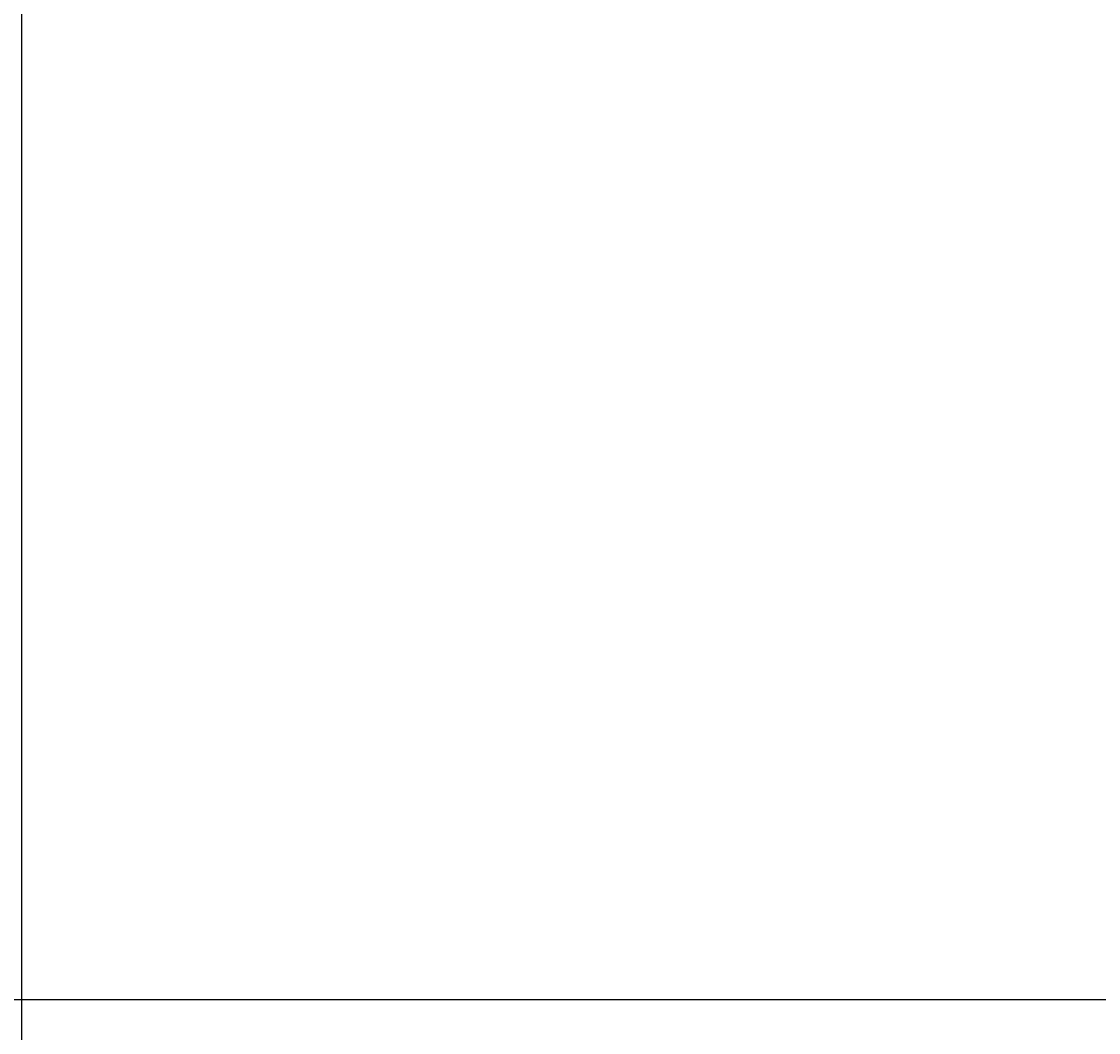
# Model space of a CAD drawing. Units: inches. Extents: x 35362 to 73946, y 43607 to 67532.
# Tile 134 of 134: x 67327 to 67834, y 59170 to 59646. Entities that reach past the tile are written whole.
import ezdxf

# ---------------------------------------------------------------- set-up
doc = ezdxf.new("R2010")
doc.units = ezdxf.units.IN
doc.header["$MEASUREMENT"] = 0
doc.layers.add('A-ANNO-DIMS', color=2, linetype='Continuous', lineweight=18)
doc.styles.get("Standard").update_dxf_attribs({"font": 'arial.ttf'})
doc.dimstyles.get("Standard").update_dxf_attribs({"dimtxt": 0.18, "dimasz": 0.18, "dimexe": 0.18, "dimexo": 0.0625, "dimgap": 0.09, "dimtad": 0, "dimtih": 1, "dimtoh": 1, "dimdec": 4, "dimzin": 0, "dimdsep": 46, "dimtxsty": 'Standard', "dimcen": 0.09, "dimadec": 0, "dimazin": 0, "dimtfac": 1, "dimtdec": 4, "dimtofl": 0, "dimtmove": 0, "dimatfit": 3, "dimfxl": 1, "dimtolj": 1, "dimtzin": 0, "dimarcsym": 0})

# ---------------------------------------------------------------- blocks, each defined once
blk = doc.blocks.new('*D8')
at = {"layer": 'A-ANNO-DIMS', "color": 0, "lineweight": -2, "transparency": 16777216}
for p, q in [((66271.28651900003, 65771.51172800003), (73945.82566600003, 65771.51172800003)), ((73945.64566600005, 65771.33172800003), (73945.64566600005, 59737.03093663782)), ((73945.64566600005, 53702.36633900002), (73945.64566600005, 59736.66713036224)), ((72185.70816600003, 53702.18633900003), (73945.82566600003, 53702.18633900003))]:
    blk.add_line(p, q, dxfattribs=at)
at = {"layer": 'A-ANNO-DIMS', "color": 0, "transparency": 16777216}
for points in [[(73945.61566600006, 65771.33172800003), (73945.67566600005, 65771.33172800003), (73945.64566600005, 65771.51172800003)], [(73945.61566600006, 53702.36633900002), (73945.67566600005, 53702.36633900002), (73945.64566600005, 53702.18633900003)]]:
    blk.add_solid(points, dxfattribs=at)
at = {"layer": 'Defpoints', "color": 0, "transparency": 16777216}
for p in [(66271.22401900003, 65771.51172800003), (73945.64566600005, 65771.51172800003), (72185.64566600003, 53702.18633900003)]:
    blk.add_point(p, dxfattribs=at)
at = {"layer": 'A-ANNO-DIMS', "color": 0, "transparency": 16777216, "insert": (73945.64566600005, 59736.84903349999), "char_height": 0.18, "attachment_point": 5}
blk.add_mtext('\\A1;12069', dxfattribs=at)
blk = doc.blocks.new('*D10')
at = {"layer": 'A-ANNO-DIMS', "color": 0, "lineweight": -2, "transparency": 16777216}
for p, q in [((61240.96983600002, 59185.14395700003), (73945.82566600003, 59185.14395700003)), ((73945.64566600005, 59184.96395700003), (73945.64566600005, 56268.51827402935)), ((73945.64566600005, 53351.70866200003), (73945.64566600005, 56268.1543449707)), ((61240.96983600002, 53351.52866200003), (73945.82566600003, 53351.52866200003))]:
    blk.add_line(p, q, dxfattribs=at)
at = {"layer": 'A-ANNO-DIMS', "color": 0, "transparency": 16777216}
for points in [[(73945.61566600006, 59184.96395700003), (73945.67566600005, 59184.96395700003), (73945.64566600005, 59185.14395700003)], [(73945.61566600006, 53351.70866200003), (73945.67566600005, 53351.70866200003), (73945.64566600005, 53351.52866200003)]]:
    blk.add_solid(points, dxfattribs=at)
at = {"layer": 'Defpoints', "color": 0, "transparency": 16777216}
for p in [(61240.90733600002, 59185.14395700003), (61240.90733600002, 53351.52866200003), (73945.64566600005, 53351.52866200003)]:
    blk.add_point(p, dxfattribs=at)
at = {"layer": 'A-ANNO-DIMS', "color": 0, "transparency": 16777216, "insert": (73945.64566600005, 56268.33630949999), "char_height": 0.18, "attachment_point": 5}
blk.add_mtext('\\A1;5834', dxfattribs=at)
blk = doc.blocks.new('*D35')
at = {"layer": 'A-ANNO-DIMS', "color": 0, "lineweight": -2, "transparency": 16777216}
for p, q in [((61240.907336, 59185.206457), (61240.907336, 67531.691728)), ((61241.08733599999, 67531.51172799998), (64780.42646373397, 67531.51172799998)), ((68320.69076200001, 67531.51172799998), (64781.35163426603, 67531.51172799998)), ((68320.870762, 60122.408832), (68320.870762, 67531.691728))]:
    blk.add_line(p, q, dxfattribs=at)
at = {"layer": 'A-ANNO-DIMS', "color": 0, "transparency": 16777216}
for points in [[(61241.08733599999, 67531.541728), (61241.08733599999, 67531.481728), (61240.907336, 67531.51172799998)], [(68320.69076200001, 67531.541728), (68320.69076200001, 67531.481728), (68320.870762, 67531.51172799998)]]:
    blk.add_solid(points, dxfattribs=at)
at = {"layer": 'Defpoints', "color": 0, "transparency": 16777216}
for p in [(68320.870762, 67531.51172799998), (68320.870762, 60122.346332), (61240.907336, 59185.14395699999)]:
    blk.add_point(p, dxfattribs=at)
at = {"layer": 'A-ANNO-DIMS', "color": 0, "transparency": 16777216, "insert": (64780.889049, 67531.51172799998), "char_height": 0.18, "attachment_point": 5}
blk.add_mtext('\\A1;7080.0', dxfattribs=at)
blk = doc.blocks.new('*D36')
at = {"layer": 'A-ANNO-DIMS', "color": 0, "lineweight": -2, "transparency": 16777216}
for p, q in [((68320.80826200004, 60122.34633200002), (35361.76908500003, 60122.34633200002)), ((35361.94908500003, 60122.16633200002), (35361.94908500003, 57247.82893113781)), ((35361.94908500003, 54373.12772400002), (35361.94908500003, 57247.46512486223)), ((68320.80826200004, 54372.94772400003), (35361.76908500003, 54372.94772400002))]:
    blk.add_line(p, q, dxfattribs=at)
at = {"layer": 'A-ANNO-DIMS', "color": 0, "transparency": 16777216}
for points in [[(35361.91908500003, 60122.16633200002), (35361.97908500003, 60122.16633200002), (35361.94908500003, 60122.34633200002)], [(35361.91908500003, 54373.12772400002), (35361.97908500003, 54373.12772400002), (35361.94908500003, 54372.94772400002)]]:
    blk.add_solid(points, dxfattribs=at)
at = {"layer": 'Defpoints', "color": 0, "transparency": 16777216}
for p in [(68320.87076200004, 60122.34633200002), (35361.94908500003, 54372.94772400002), (68320.87076200004, 54372.94772400003)]:
    blk.add_point(p, dxfattribs=at)
at = {"layer": 'A-ANNO-DIMS', "color": 0, "transparency": 16777216, "insert": (35361.94908500004, 57247.64702799999), "char_height": 0.18, "attachment_point": 5}
blk.add_mtext('\\A1;5749.4', dxfattribs=at)
blk = doc.blocks.new('*D65')
at = {"layer": 'A-ANNO-DIMS', "color": 0, "lineweight": -2, "transparency": 16777216}
for p, q in [((65336.01600799999, 61293.223552), (65336.01600799999, 43606.678996)), ((67326.639741, 61293.223552), (67326.639741, 43606.678996)), ((65336.19600799999, 43606.858996), (66330.87277900206, 43606.858996)), ((67326.45974100001, 43606.858996), (66331.78296999796, 43606.858996))]:
    blk.add_line(p, q, dxfattribs=at)
at = {"layer": 'A-ANNO-DIMS', "color": 0, "transparency": 16777216}
for points in [[(65336.19600799999, 43606.888996), (65336.19600799999, 43606.828996), (65336.01600799999, 43606.858996)], [(67326.45974100001, 43606.888996), (67326.45974100001, 43606.828996), (67326.639741, 43606.858996)]]:
    blk.add_solid(points, dxfattribs=at)
at = {"layer": 'Defpoints', "color": 0, "transparency": 16777216}
for p in [(65336.01600799999, 61293.286052), (67326.639741, 61293.286052), (67326.639741, 43606.858996)]:
    blk.add_point(p, dxfattribs=at)
at = {"layer": 'A-ANNO-DIMS', "color": 0, "transparency": 16777216, "insert": (66331.32787450001, 43606.858996), "char_height": 0.18, "attachment_point": 5}
blk.add_mtext('\\A1;1990.6', dxfattribs=at)
blk = doc.blocks.new('*D70')
at = {"layer": 'A-ANNO-DIMS', "color": 0, "lineweight": -2, "transparency": 16777216}
for p, q in [((60785.27513900002, 64923.75242000003), (73945.82566600003, 64923.75242000003)), ((73945.64566600005, 64923.57242000003), (73945.64566600005, 62054.63015302935)), ((73945.64566600005, 59185.32395700003), (73945.64566600005, 62054.26622397069)), ((61240.96983600002, 59185.14395700003), (73945.82566600003, 59185.14395700003))]:
    blk.add_line(p, q, dxfattribs=at)
at = {"layer": 'A-ANNO-DIMS', "color": 0, "transparency": 16777216}
for points in [[(73945.61566600006, 64923.57242000003), (73945.67566600005, 64923.57242000003), (73945.64566600005, 64923.75242000003)], [(73945.61566600006, 59185.32395700003), (73945.67566600005, 59185.32395700003), (73945.64566600005, 59185.14395700003)]]:
    blk.add_solid(points, dxfattribs=at)
at = {"layer": 'Defpoints', "color": 0, "transparency": 16777216}
for p in [(60785.21263900002, 64923.75242000003), (73945.64566600005, 64923.75242000003), (61240.90733600002, 59185.14395700003)]:
    blk.add_point(p, dxfattribs=at)
at = {"layer": 'A-ANNO-DIMS', "color": 0, "transparency": 16777216, "insert": (73945.64566600005, 62054.44818849999), "char_height": 0.18, "attachment_point": 5}
blk.add_mtext('\\A1;5738.6', dxfattribs=at)
blk = doc.blocks.new('*D71')
at = {"layer": 'A-ANNO-DIMS', "color": 0, "lineweight": -2, "transparency": 16777216}
for p, q in [((63159.24181700003, 64828.55626700002), (73945.82566600003, 64828.55626700002)), ((73945.64566600005, 64828.37626700002), (73945.64566600005, 62007.03207652936)), ((73945.64566600005, 59185.32395700003), (73945.64566600005, 62006.6681474707)), ((61240.96983600002, 59185.14395700003), (73945.82566600003, 59185.14395700003))]:
    blk.add_line(p, q, dxfattribs=at)
at = {"layer": 'A-ANNO-DIMS', "color": 0, "transparency": 16777216}
for points in [[(73945.61566600006, 64828.37626700002), (73945.67566600005, 64828.37626700002), (73945.64566600005, 64828.55626700002)], [(73945.61566600006, 59185.32395700003), (73945.67566600005, 59185.32395700003), (73945.64566600005, 59185.14395700003)]]:
    blk.add_solid(points, dxfattribs=at)
at = {"layer": 'Defpoints', "color": 0, "transparency": 16777216}
for p in [(63159.17931700003, 64828.55626700002), (73945.64566600005, 64828.55626700002), (61240.90733600002, 59185.14395700003)]:
    blk.add_point(p, dxfattribs=at)
at = {"layer": 'A-ANNO-DIMS', "color": 0, "transparency": 16777216, "insert": (73945.64566600005, 62006.85011199999), "char_height": 0.18, "attachment_point": 5}
blk.add_mtext('\\A1;5643.4', dxfattribs=at)

msp = doc.modelspace()

# ---------------------------------------------------------------- dimensions: what is measured, and where the dimension line sits
at = {"layer": 'A-ANNO-DIMS'}
for base, p1, p2, picture, middle in [((68320.870762, 67531.51172799998), (61240.907336, 59185.14395699999), (68320.870762, 60122.346332), '*D35', (64780.889049, 67531.51172799998)), ((67326.639741, 43606.858996), (65336.01600799999, 61293.286052), (67326.639741, 61293.286052), '*D65', (66331.32787450001, 43606.858996))]:
    dim = msp.add_linear_dim(base=base, p1=p1, p2=p2, dimstyle='Standard', override={"dimdec": 1, "dimlfac": 1, "dimrnd": 0, "dimzin": 0, "dimdsep": 46, "dimlunit": 2}, dxfattribs=at)
    dim.commit()
    dim.dimension.update_dxf_attribs({"geometry": picture, "text_midpoint": middle})
for base, p1, p2, override, picture, middle in [((73945.64566600005, 65771.51172800003), (72185.645666, 53702.186339), (66271.224019, 65771.51172799998), {"dimdec": 0, "dimlfac": 1, "dimrnd": 0, "dimzin": 0, "dimdsep": 46, "dimlunit": 2}, '*D8', (73945.64566600005, 59736.84903349999)), ((73945.64566600005, 64923.75242000003), (61240.907336, 59185.14395699999), (60785.21263899999, 64923.75241999999), {"dimdec": 1, "dimlfac": 1, "dimrnd": 0, "dimzin": 0, "dimdsep": 46, "dimlunit": 2}, '*D70', (73945.64566600005, 62054.44818849999)), ((73945.64566600005, 64828.55626700002), (61240.907336, 59185.14395699999), (63159.179317, 64828.556267), {"dimdec": 1, "dimlfac": 1, "dimrnd": 0, "dimzin": 0, "dimdsep": 46, "dimlunit": 2}, '*D71', (73945.64566600005, 62006.85011199999)), ((35361.94908500003, 54372.94772400002), (68320.870762, 60122.346332), (68320.870762, 54372.947724), {"dimdec": 1, "dimlfac": 1, "dimrnd": 0, "dimzin": 0, "dimdsep": 46, "dimlunit": 2}, '*D36', (35361.94908500004, 57247.64702799999)), ((73945.64566600005, 53351.52866200003), (61240.907336, 59185.14395699999), (61240.907336, 53351.52866199999), {"dimdec": 0, "dimlfac": 1, "dimrnd": 0, "dimzin": 0, "dimdsep": 46, "dimlunit": 2}, '*D10', (73945.64566600005, 56268.33630949999))]:
    dim = msp.add_linear_dim(base=base, p1=p1, p2=p2, angle=90, dimstyle='Standard', override=override, dxfattribs=at)
    dim.commit()
    dim.dimension.update_dxf_attribs({"geometry": picture, "text_midpoint": middle})

doc.saveas('drawing.dxf')
